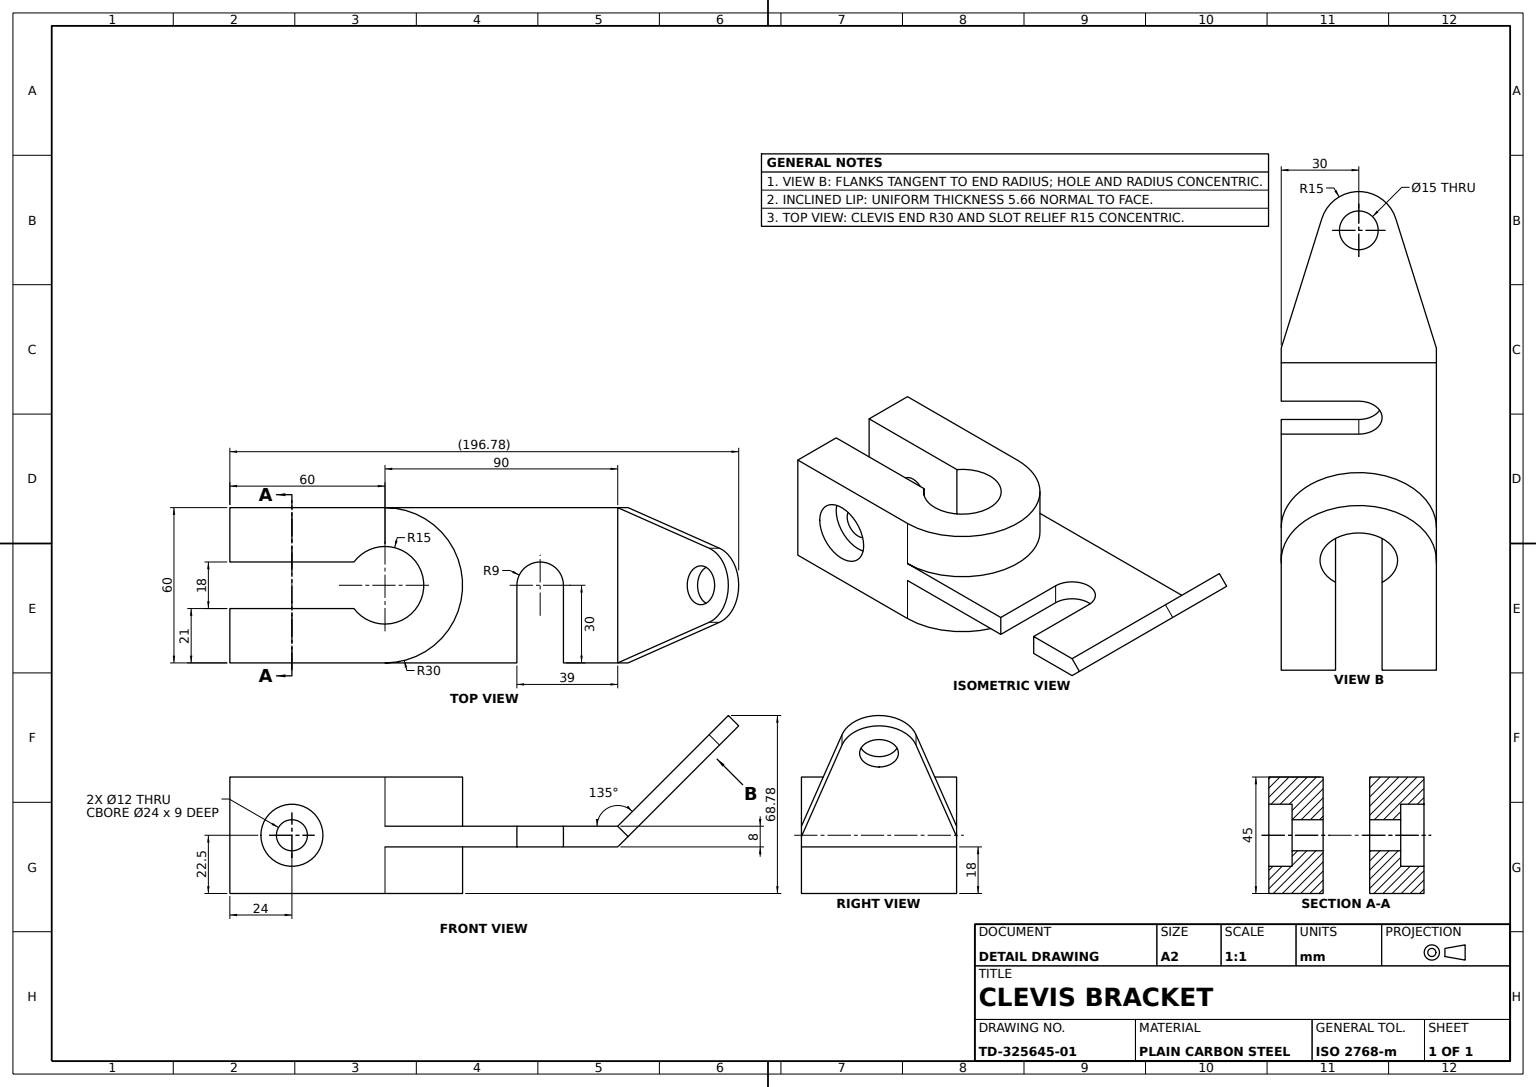
SolidWorks part; units mm, degrees
material "Plain Carbon Steel"
ref_plane "Front Plane" through (0, 0, 0) normal (0, 0, 1) x (1, 0, 0)
ref_plane "Top Plane" through (0, 0, 0) normal (0, 1, 0) x (1, 0, 0)
ref_plane "Right Plane" through (0, 0, 0) normal (1, 0, 0) x (0, 0, -1)
sketch "Base Block Sketch" plane through (0, 0, 0) normal (0, 1, 0) x (1, 0, 0)
  line L0 (-61.4501, 0) -> (62.866, 0) construction
  line L1 (-60, 9) -> (-12, 9)
  line L2 (-60, -9) -> (-12, -9)
  line L3 (0, 46.6908) -> (0, -40.9003) construction
  line L4 (0, 30) -> (-60, 30)
  line L5 (0, -30) -> (-60, -30)
  line L6 (-60, 30) -> (-60, -30)
  arc A0 (-12, -9) -> (-12, 9) centre (0, 0) ccw
  arc A1 (0, -30) -> (0, 30) centre (0, 0) ccw
  dimension "D1" = 30
  dimension "D2" = 60
  dimension "D3" = 18
  dimension "D4" = 60
extrude "Base Block" add sketch "Base Block Sketch" along normal blind 45 contours L5 A1 L4 L6 L1 A0 L2
ref_plane "Tab Plane" through (0, 18, 0) normal (0, -1, 0) x (-1, 0, 0)
sketch "Slotted Tab Sketch" plane through (0, 18, 0) normal (0, -1, 0) x (-1, 0, 0)
  line L0 (-139.7938, 0) -> (-69, 0) construction
  line L1 (0, 90.6785) -> (0, -76.132) construction
  line L2 (0, 30) -> (-51, 30)
  line L3 (0, -30) -> (-51, -30)
  line L4 (-69, 0) -> (-69, -30)
  line L5 (-51, 0) -> (-51, -30)
  line L6 (-90, 30) -> (-90, -30)
  line L7 (-69, -30) -> (-90, -30)
  line L8 (-51, 30) -> (-90, 30)
  line L9 (-51, 0) -> (118.881, 0) construction
  arc A2 (0, 30) -> (0, -30) centre (0, 0) ccw construction
  arc A3 (0, 30) -> (0, -30) centre (0, 0) ccw
  arc A4 (-51, 0) -> (-69, 0) centre (-60, 0) ccw
  dimension "D2" = 9
  dimension "D1" = 90
  dimension "D3" = 39
extrude "Slotted Tab" add sketch "Slotted Tab Sketch" against normal blind 8
sketch "Angled Lip Sketch" plane through (0, 0, 30) normal (0, 0, 1) x (1, 0, 0)
  line L1 (90, 18) -> (137, 65)
  line L2 (90, 26) -> (90, 18) construction
  line L4 (90, 26) -> (133, 69)
  line L5 (137, 65) -> (133, 69)
  line L6 (90, 18) -> (90, 26)
  line L7 (90, 26) -> (69, 26) construction
  dimension "D1" = 43
  dimension "D3" = 135
extrude "Angled Lip" add sketch "Angled Lip Sketch" against normal up to surface (60 mm away) up to face at (7.5, 22.25, -30)
sketch "Clevis Slot Sketch" plane through (32, -32, 0) normal (-0.7071, 0.7071, 0) x (0, 0, 1)
  line L0 (0, 82.0244) -> (0, 168.1277) construction
  line L1 (-30, 82.0244) -> (30, 82.0244) construction
  line L3 (-14.3118, 132.0157) -> (-30, 82.0244)
  line L4 (14.3118, 132.0157) -> (30, 82.0244)
  line L6 (-33.8128, 82.0244) -> (-30, 82.0244)
  line L8 (-33.8128, 82.0244) -> (-33.8128, 155.3192)
  line L9 (-33.8128, 155.3192) -> (36.024, 155.3192)
  line L10 (36.024, 82.0244) -> (36.024, 155.3192)
  line L11 (30, 82.0244) -> (36.024, 82.0244)
  arc A0 (14.3118, 132.0157) -> (-14.3118, 132.0157) centre (0, 127.5244) ccw
  point P9 (0, 112.5244)
  dimension "D2" = 15
  dimension "D3" = 66.024
  dimension "D1" = 45.5
  dimension "D4" = 3.8128
  dimension "D5" = 73.2948
extrude "Clevis Slot" cut sketch "Clevis Slot Sketch" against normal blind 9
hole_wizard "Clevis Cross Hole M14 Ø15" positions "Sketch8" profile "Sketch7" hole size "M14" standard "ANSI Metric" end condition up to next
sketch "Sketch8" plane through (32, -32, 0) normal (-0.7071, 0.7071, 0) x (0.7071, 0.7071, 0)
  point P0 (127.5244, 0)
sketch "Sketch7" plane through (122.1734, 58.1734, 0) normal (0, 0, 1) x (-0.7071, -0.7071, 0)
  line L0 (0, 0) -> (0, 5.6569)
  line L1 (0, 5.6569) -> (7.5, 5.6569)
  line L2 (7.5, 5.6569) -> (7.5, 0)
  line L5 (7.5, 0) -> (0, 0)
  line L11 (0, -6.35) -> (0, 107.95) construction
  dimension "Thru Hole Dia." = 15
  dimension "Thru Hole Depth" = 5.6569
hole_wizard "Counterbored Bolt Hole M10" positions "Sketch9" profile "Sketch10" counterbore size "M10" standard "ANSI Metric"
sketch "Sketch9" plane through (0, 0, 30) normal (0, 0, 1) x (1, 0, 0)
  line L0 (0, 0) -> (-60, 0) construction
  line L1 (-60, 45) -> (-60, 0) construction
  point P0 (-36, 22.5)
  dimension "D1" = 22.5
  dimension "D2" = 24
sketch "Sketch10" plane through (-36, 22.5, 30) normal (1, 0, 0) x (0, -1, 0)
  line L0 (0, 0) -> (0, 21)
  line L1 (0, 21) -> (6, 21)
  line L3 (6, 21) -> (6, 9)
  line L4 (6, 9) -> (12, 9)
  line L5 (12, 9) -> (12, 0)
  line L7 (12, 0) -> (0, 0)
  line L11 (0, -6.35) -> (0, 107.95) construction
  dimension "Thru Hole Dia." = 12
  dimension "Thru Hole Depth" = 21
  dimension "C'Bore Dia." = 24
  dimension "C'Bore Depth" = 9
mirror "Bolt Hole Mirror" about plane through (0, 0, 0) normal (0, 0, 1) of "Counterbored Bolt Hole M10"
